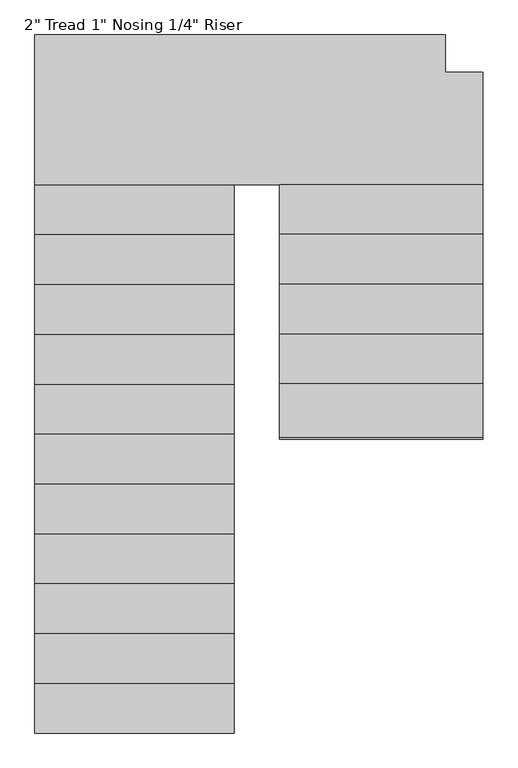
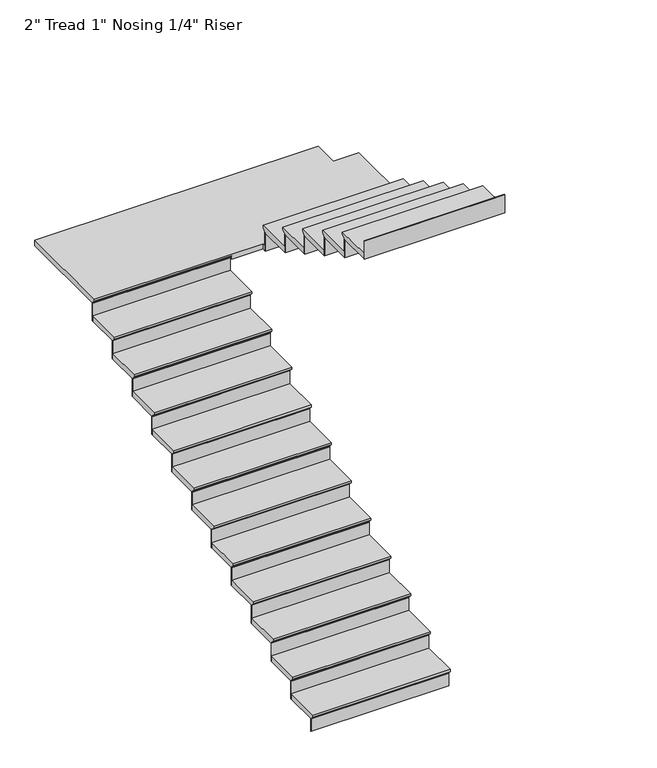
"""IFC4 building model written with IfcOpenShell, lengths in millimetres: stair flight geometry."""

from ifc_helpers import new_model, si_unit, origin, place, context, project, spatial, faceted_brep, source, transform, mapped, element, save


def stair_flight_991562f7(model_context):
    return source(origin(), model_context, "Body", "Brep", [
        faceted_brep([(-1810.3456086, -4300.9794704, 6551.0833333), (-1810.3456086, -4300.9794704, 6570.1333333), (-3029.5456086, -4300.9794704, 6570.1333333), (-3029.5456086, -4300.9794704, 6551.0833333), (-1810.3456086, -4275.5794704, 6525.6833333), (-3029.5456086, -4275.5794704, 6525.6833333), (-1810.3456086, -3970.7794704, 6570.1333333), (-3029.5456086, -3970.7794704, 6570.1333333), (-3029.5456086, -4275.5794704, 6519.3333333), (-3029.5456086, -3970.7794704, 6519.3333333), (-1810.3456086, -3970.7794704, 6519.3333333), (-1810.3456086, -4275.5794704, 6519.3333333)], [[[0, 1, 2, 3]], [[4, 0, 3, 5]], [[2, 1, 6, 7]], [[8, 9, 10, 11]], [[2, 7, 9, 8, 5, 3]], [[8, 11, 4, 5]], [[6, 1, 0, 4, 11, 10]], [[7, 6, 10, 9]]]),
        faceted_brep([(-1810.3456086, -4275.5794704, 6519.3333333), (-1810.3456086, -4275.5794704, 6400.8), (-1810.3456086, -4269.2294704, 6400.8), (-1810.3456086, -4269.2294704, 6519.3333333), (-3029.5456086, -4275.5794704, 6519.3333333), (-3029.5456086, -4269.2294704, 6519.3333333), (-3029.5456086, -4269.2294704, 6400.8), (-3029.5456086, -4275.5794704, 6400.8)], [[[0, 1, 2, 3]], [[4, 5, 6, 7]], [[1, 0, 4, 7]], [[2, 1, 7, 6]], [[3, 2, 6, 5]], [[0, 3, 5, 4]]]),
        faceted_brep([(-1810.3456086, -3970.7794704, 6688.6666667), (-1810.3456086, -3970.7794704, 6519.3333333), (-1810.3456086, -3964.4294704, 6519.3333333), (-1810.3456086, -3964.4294704, 6688.6666667), (-3029.5456086, -3970.7794704, 6688.6666667), (-3029.5456086, -3964.4294704, 6688.6666667), (-3029.5456086, -3964.4294704, 6519.3333333), (-3029.5456086, -3970.7794704, 6519.3333333)], [[[0, 1, 2, 3]], [[4, 5, 6, 7]], [[1, 0, 4, 7]], [[2, 1, 7, 6]], [[3, 2, 6, 5]], [[0, 3, 5, 4]]]),
        faceted_brep([(-3029.5456086, -3996.1794704, 6739.4666667), (-1810.3456086, -3996.1794704, 6739.4666667), (-1810.3456086, -3665.9794704, 6739.4666667), (-3029.5456086, -3665.9794704, 6739.4666667), (-3029.5456086, -3970.7794704, 6688.6666667), (-3029.5456086, -3665.9794704, 6688.6666667), (-1810.3456086, -3665.9794704, 6688.6666667), (-1810.3456086, -3970.7794704, 6688.6666667), (-3029.5456086, -3970.7794704, 6695.0166667), (-3029.5456086, -3996.1794704, 6720.4166667), (-1810.3456086, -3970.7794704, 6695.0166667), (-1810.3456086, -3996.1794704, 6720.4166667)], [[[0, 1, 2, 3]], [[4, 5, 6, 7]], [[0, 3, 5, 4, 8, 9]], [[4, 7, 10, 8]], [[2, 1, 11, 10, 7, 6]], [[3, 2, 6, 5]], [[11, 1, 0, 9]], [[10, 11, 9, 8]]]),
        faceted_brep([(-1810.3456086, -3665.9794704, 6858.0), (-1810.3456086, -3665.9794704, 6688.6666667), (-1810.3456086, -3659.6294704, 6688.6666667), (-1810.3456086, -3659.6294704, 6858.0), (-3029.5456086, -3665.9794704, 6858.0), (-3029.5456086, -3659.6294704, 6858.0), (-3029.5456086, -3659.6294704, 6688.6666667), (-3029.5456086, -3665.9794704, 6688.6666667)], [[[0, 1, 2, 3]], [[4, 5, 6, 7]], [[1, 0, 4, 7]], [[2, 1, 7, 6]], [[3, 2, 6, 5]], [[0, 3, 5, 4]]]),
        faceted_brep([(-3029.5456086, -3691.3794704, 6908.8), (-1810.3456086, -3691.3794704, 6908.8), (-1810.3456086, -3361.1794704, 6908.8), (-3029.5456086, -3361.1794704, 6908.8), (-3029.5456086, -3665.9794704, 6858.0), (-3029.5456086, -3361.1794704, 6858.0), (-1810.3456086, -3361.1794704, 6858.0), (-1810.3456086, -3665.9794704, 6858.0), (-3029.5456086, -3665.9794704, 6864.35), (-3029.5456086, -3691.3794704, 6889.75), (-1810.3456086, -3665.9794704, 6864.35), (-1810.3456086, -3691.3794704, 6889.75)], [[[0, 1, 2, 3]], [[4, 5, 6, 7]], [[0, 3, 5, 4, 8, 9]], [[4, 7, 10, 8]], [[2, 1, 11, 10, 7, 6]], [[3, 2, 6, 5]], [[11, 1, 0, 9]], [[10, 11, 9, 8]]]),
        faceted_brep([(-1810.3456086, -3361.1794704, 7027.3333333), (-1810.3456086, -3361.1794704, 6858.0), (-1810.3456086, -3354.8294704, 6858.0), (-1810.3456086, -3354.8294704, 7027.3333333), (-3029.5456086, -3361.1794704, 7027.3333333), (-3029.5456086, -3354.8294704, 7027.3333333), (-3029.5456086, -3354.8294704, 6858.0), (-3029.5456086, -3361.1794704, 6858.0)], [[[0, 1, 2, 3]], [[4, 5, 6, 7]], [[1, 0, 4, 7]], [[2, 1, 7, 6]], [[3, 2, 6, 5]], [[0, 3, 5, 4]]]),
        faceted_brep([(-3029.5456086, -3386.5794704, 7078.1333333), (-1810.3456086, -3386.5794704, 7078.1333333), (-1810.3456086, -3056.3794704, 7078.1333333), (-3029.5456086, -3056.3794704, 7078.1333333), (-3029.5456086, -3361.1794704, 7027.3333333), (-3029.5456086, -3056.3794704, 7027.3333333), (-1810.3456086, -3056.3794704, 7027.3333333), (-1810.3456086, -3361.1794704, 7027.3333333), (-3029.5456086, -3361.1794704, 7033.6833333), (-3029.5456086, -3386.5794704, 7059.0833333), (-1810.3456086, -3361.1794704, 7033.6833333), (-1810.3456086, -3386.5794704, 7059.0833333)], [[[0, 1, 2, 3]], [[4, 5, 6, 7]], [[0, 3, 5, 4, 8, 9]], [[4, 7, 10, 8]], [[2, 1, 11, 10, 7, 6]], [[3, 2, 6, 5]], [[11, 1, 0, 9]], [[10, 11, 9, 8]]]),
        faceted_brep([(-1810.3456086, -3056.3794704, 7196.6666667), (-1810.3456086, -3056.3794704, 7027.3333333), (-1810.3456086, -3050.0294704, 7027.3333333), (-1810.3456086, -3050.0294704, 7196.6666667), (-3029.5456086, -3056.3794704, 7196.6666667), (-3029.5456086, -3050.0294704, 7196.6666667), (-3029.5456086, -3050.0294704, 7027.3333333), (-3029.5456086, -3056.3794704, 7027.3333333)], [[[0, 1, 2, 3]], [[4, 5, 6, 7]], [[1, 0, 4, 7]], [[2, 1, 7, 6]], [[3, 2, 6, 5]], [[0, 3, 5, 4]]]),
        faceted_brep([(-3029.5456086, -3081.7794704, 7247.4666667), (-1810.3456086, -3081.7794704, 7247.4666667), (-1810.3456086, -2751.5794704, 7247.4666667), (-3029.5456086, -2751.5794704, 7247.4666667), (-3029.5456086, -3056.3794704, 7196.6666667), (-3029.5456086, -2751.5794704, 7196.6666667), (-1810.3456086, -2751.5794704, 7196.6666667), (-1810.3456086, -3056.3794704, 7196.6666667), (-3029.5456086, -3056.3794704, 7203.0166667), (-3029.5456086, -3081.7794704, 7228.4166667), (-1810.3456086, -3056.3794704, 7203.0166667), (-1810.3456086, -3081.7794704, 7228.4166667)], [[[0, 1, 2, 3]], [[4, 5, 6, 7]], [[0, 3, 5, 4, 8, 9]], [[4, 7, 10, 8]], [[2, 1, 11, 10, 7, 6]], [[3, 2, 6, 5]], [[11, 1, 0, 9]], [[10, 11, 9, 8]]]),
        faceted_brep([(-1810.3456086, -2751.5794704, 7366.0), (-1810.3456086, -2751.5794704, 7196.6666667), (-1810.3456086, -2745.2294704, 7196.6666667), (-1810.3456086, -2745.2294704, 7366.0), (-3029.5456086, -2751.5794704, 7366.0), (-3029.5456086, -2745.2294704, 7366.0), (-3029.5456086, -2745.2294704, 7196.6666667), (-3029.5456086, -2751.5794704, 7196.6666667)], [[[0, 1, 2, 3]], [[4, 5, 6, 7]], [[1, 0, 4, 7]], [[2, 1, 7, 6]], [[3, 2, 6, 5]], [[0, 3, 5, 4]]]),
        faceted_brep([(-3029.5456086, -2776.9794704, 7416.8), (-1810.3456086, -2776.9794704, 7416.8), (-1810.3456086, -2446.7794704, 7416.8), (-3029.5456086, -2446.7794704, 7416.8), (-3029.5456086, -2751.5794704, 7366.0), (-3029.5456086, -2446.7794704, 7366.0), (-1810.3456086, -2446.7794704, 7366.0), (-1810.3456086, -2751.5794704, 7366.0), (-3029.5456086, -2751.5794704, 7372.35), (-3029.5456086, -2776.9794704, 7397.75), (-1810.3456086, -2751.5794704, 7372.35), (-1810.3456086, -2776.9794704, 7397.75)], [[[0, 1, 2, 3]], [[4, 5, 6, 7]], [[0, 3, 5, 4, 8, 9]], [[4, 7, 10, 8]], [[2, 1, 11, 10, 7, 6]], [[3, 2, 6, 5]], [[11, 1, 0, 9]], [[10, 11, 9, 8]]]),
        faceted_brep([(-1810.3456086, -2446.7794704, 7535.3333333), (-1810.3456086, -2446.7794704, 7366.0), (-1810.3456086, -2440.4294704, 7366.0), (-1810.3456086, -2440.4294704, 7535.3333333), (-3029.5456086, -2446.7794704, 7535.3333333), (-3029.5456086, -2440.4294704, 7535.3333333), (-3029.5456086, -2440.4294704, 7366.0), (-3029.5456086, -2446.7794704, 7366.0)], [[[0, 1, 2, 3]], [[4, 5, 6, 7]], [[1, 0, 4, 7]], [[2, 1, 7, 6]], [[3, 2, 6, 5]], [[0, 3, 5, 4]]]),
        faceted_brep([(-3029.5456086, -2472.1794704, 7586.1333333), (-1810.3456086, -2472.1794704, 7586.1333333), (-1810.3456086, -2141.9794704, 7586.1333333), (-3029.5456086, -2141.9794704, 7586.1333333), (-3029.5456086, -2446.7794704, 7535.3333333), (-3029.5456086, -2141.9794704, 7535.3333333), (-1810.3456086, -2141.9794704, 7535.3333333), (-1810.3456086, -2446.7794704, 7535.3333333), (-3029.5456086, -2446.7794704, 7541.6833333), (-3029.5456086, -2472.1794704, 7567.0833333), (-1810.3456086, -2446.7794704, 7541.6833333), (-1810.3456086, -2472.1794704, 7567.0833333)], [[[0, 1, 2, 3]], [[4, 5, 6, 7]], [[0, 3, 5, 4, 8, 9]], [[4, 7, 10, 8]], [[2, 1, 11, 10, 7, 6]], [[3, 2, 6, 5]], [[11, 1, 0, 9]], [[10, 11, 9, 8]]]),
        faceted_brep([(-1810.3456086, -2141.9794704, 7704.6666667), (-1810.3456086, -2141.9794704, 7535.3333333), (-1810.3456086, -2135.6294704, 7535.3333333), (-1810.3456086, -2135.6294704, 7704.6666667), (-3029.5456086, -2141.9794704, 7704.6666667), (-3029.5456086, -2135.6294704, 7704.6666667), (-3029.5456086, -2135.6294704, 7535.3333333), (-3029.5456086, -2141.9794704, 7535.3333333)], [[[0, 1, 2, 3]], [[4, 5, 6, 7]], [[1, 0, 4, 7]], [[2, 1, 7, 6]], [[3, 2, 6, 5]], [[0, 3, 5, 4]]]),
        faceted_brep([(-3029.5456086, -2167.3794704, 7755.4666667), (-1810.3456086, -2167.3794704, 7755.4666667), (-1810.3456086, -1837.1794704, 7755.4666667), (-3029.5456086, -1837.1794704, 7755.4666667), (-3029.5456086, -2141.9794704, 7704.6666667), (-3029.5456086, -1837.1794704, 7704.6666667), (-1810.3456086, -1837.1794704, 7704.6666667), (-1810.3456086, -2141.9794704, 7704.6666667), (-3029.5456086, -2141.9794704, 7711.0166667), (-3029.5456086, -2167.3794704, 7736.4166667), (-1810.3456086, -2141.9794704, 7711.0166667), (-1810.3456086, -2167.3794704, 7736.4166667)], [[[0, 1, 2, 3]], [[4, 5, 6, 7]], [[0, 3, 5, 4, 8, 9]], [[4, 7, 10, 8]], [[2, 1, 11, 10, 7, 6]], [[3, 2, 6, 5]], [[11, 1, 0, 9]], [[10, 11, 9, 8]]]),
        faceted_brep([(-1810.3456086, -1837.1794704, 7874.0), (-1810.3456086, -1837.1794704, 7704.6666667), (-1810.3456086, -1830.8294704, 7704.6666667), (-1810.3456086, -1830.8294704, 7874.0), (-3029.5456086, -1837.1794704, 7874.0), (-3029.5456086, -1830.8294704, 7874.0), (-3029.5456086, -1830.8294704, 7704.6666667), (-3029.5456086, -1837.1794704, 7704.6666667)], [[[0, 1, 2, 3]], [[4, 5, 6, 7]], [[1, 0, 4, 7]], [[2, 1, 7, 6]], [[3, 2, 6, 5]], [[0, 3, 5, 4]]]),
        faceted_brep([(-3029.5456086, -1862.5794704, 7924.8), (-1810.3456086, -1862.5794704, 7924.8), (-1810.3456086, -1532.3794704, 7924.8), (-3029.5456086, -1532.3794704, 7924.8), (-3029.5456086, -1837.1794704, 7874.0), (-3029.5456086, -1532.3794704, 7874.0), (-1810.3456086, -1532.3794704, 7874.0), (-1810.3456086, -1837.1794704, 7874.0), (-3029.5456086, -1837.1794704, 7880.35), (-3029.5456086, -1862.5794704, 7905.75), (-1810.3456086, -1837.1794704, 7880.35), (-1810.3456086, -1862.5794704, 7905.75)], [[[0, 1, 2, 3]], [[4, 5, 6, 7]], [[0, 3, 5, 4, 8, 9]], [[4, 7, 10, 8]], [[2, 1, 11, 10, 7, 6]], [[3, 2, 6, 5]], [[11, 1, 0, 9]], [[10, 11, 9, 8]]]),
        faceted_brep([(-1810.3456086, -1532.3794704, 8043.3333333), (-1810.3456086, -1532.3794704, 7874.0), (-1810.3456086, -1526.0294704, 7874.0), (-1810.3456086, -1526.0294704, 8043.3333333), (-3029.5456086, -1532.3794704, 8043.3333333), (-3029.5456086, -1526.0294704, 8043.3333333), (-3029.5456086, -1526.0294704, 7874.0), (-3029.5456086, -1532.3794704, 7874.0)], [[[0, 1, 2, 3]], [[4, 5, 6, 7]], [[1, 0, 4, 7]], [[2, 1, 7, 6]], [[3, 2, 6, 5]], [[0, 3, 5, 4]]]),
        faceted_brep([(-3029.5456086, -1557.7794704, 8094.1333333), (-1810.3456086, -1557.7794704, 8094.1333333), (-1810.3456086, -1227.5794704, 8094.1333333), (-3029.5456086, -1227.5794704, 8094.1333333), (-3029.5456086, -1532.3794704, 8043.3333333), (-3029.5456086, -1227.5794704, 8043.3333333), (-1810.3456086, -1227.5794704, 8043.3333333), (-1810.3456086, -1532.3794704, 8043.3333333), (-3029.5456086, -1532.3794704, 8049.6833333), (-3029.5456086, -1557.7794704, 8075.0833333), (-1810.3456086, -1532.3794704, 8049.6833333), (-1810.3456086, -1557.7794704, 8075.0833333)], [[[0, 1, 2, 3]], [[4, 5, 6, 7]], [[0, 3, 5, 4, 8, 9]], [[4, 7, 10, 8]], [[2, 1, 11, 10, 7, 6]], [[3, 2, 6, 5]], [[11, 1, 0, 9]], [[10, 11, 9, 8]]]),
        faceted_brep([(-1810.3456086, -1227.5794704, 8212.6666667), (-1810.3456086, -1227.5794704, 8043.3333333), (-1810.3456086, -1221.2294704, 8043.3333333), (-1810.3456086, -1221.2294704, 8212.6666667), (-3029.5456086, -1227.5794704, 8212.6666667), (-3029.5456086, -1221.2294704, 8212.6666667), (-3029.5456086, -1221.2294704, 8043.3333333), (-3029.5456086, -1227.5794704, 8043.3333333)], [[[0, 1, 2, 3]], [[4, 5, 6, 7]], [[1, 0, 4, 7]], [[2, 1, 7, 6]], [[3, 2, 6, 5]], [[0, 3, 5, 4]]]),
        faceted_brep([(-3029.5456086, -1252.9794704, 8263.4666667), (-1810.3456086, -1252.9794704, 8263.4666667), (-1810.3456086, -922.7794704, 8263.4666667), (-3029.5456086, -922.7794704, 8263.4666667), (-3029.5456086, -1227.5794704, 8212.6666667), (-3029.5456086, -922.7794704, 8212.6666667), (-1810.3456086, -922.7794704, 8212.6666667), (-1810.3456086, -1227.5794704, 8212.6666667), (-3029.5456086, -1227.5794704, 8219.0166667), (-3029.5456086, -1252.9794704, 8244.4166667), (-1810.3456086, -1227.5794704, 8219.0166667), (-1810.3456086, -1252.9794704, 8244.4166667)], [[[0, 1, 2, 3]], [[4, 5, 6, 7]], [[0, 3, 5, 4, 8, 9]], [[4, 7, 10, 8]], [[2, 1, 11, 10, 7, 6]], [[3, 2, 6, 5]], [[11, 1, 0, 9]], [[10, 11, 9, 8]]]),
        faceted_brep([(-1810.3456086, -922.7794704, 8382.0), (-1810.3456086, -922.7794704, 8212.6666667), (-1810.3456086, -916.4294704, 8212.6666667), (-1810.3456086, -916.4294704, 8382.0), (-3029.5456086, -922.7794704, 8382.0), (-3029.5456086, -916.4294704, 8382.0), (-3029.5456086, -916.4294704, 8212.6666667), (-3029.5456086, -922.7794704, 8212.6666667)], [[[0, 1, 2, 3]], [[4, 5, 6, 7]], [[1, 0, 4, 7]], [[2, 1, 7, 6]], [[3, 2, 6, 5]], [[0, 3, 5, 4]]]),
        faceted_brep([(-289.8083398, -973.5794704, 8432.8), (-289.8083398, -262.3794704, 8432.8), (-518.4083398, -262.3794704, 8432.8), (-518.4083398, -33.7794704, 8432.8), (-3029.5456086, -33.7794704, 8432.8), (-3029.5456086, -948.1794704, 8432.8), (-1534.4083398, -948.1794704, 8432.8), (-1534.4083398, -973.5794704, 8432.8), (-289.8083398, -262.3794704, 8382.0), (-289.8083398, -973.5794704, 8382.0), (-1534.4083398, -973.5794704, 8382.0), (-1534.4083398, -948.1794704, 8382.0), (-1810.3456086, -948.1794704, 8382.0), (-1810.3456086, -922.7794704, 8382.0), (-3029.5456086, -922.7794704, 8382.0), (-3029.5456086, -33.7794704, 8382.0), (-518.4083398, -33.7794704, 8382.0), (-518.4083398, -262.3794704, 8382.0), (-3029.5456086, -922.7794704, 8388.35), (-3029.5456086, -948.1794704, 8413.75), (-1810.3456086, -922.7794704, 8388.35), (-1810.3456086, -948.1794704, 8413.75)], [[[0, 1, 2, 3, 4, 5, 6, 7]], [[8, 9, 10, 11, 12, 13, 14, 15, 16, 17]], [[1, 0, 9, 8]], [[2, 1, 8, 17]], [[3, 2, 17, 16]], [[4, 3, 16, 15]], [[5, 4, 15, 14, 18, 19]], [[14, 13, 20, 18]], [[13, 12, 21, 20]], [[6, 5, 19, 21, 12, 11]], [[7, 6, 11, 10]], [[0, 7, 10, 9]], [[19, 18, 20, 21]]]),
        faceted_brep([(-1534.4083398, -973.5794704, 8551.3333333), (-1534.4083398, -973.5794704, 8382.0), (-1534.4083398, -979.9294704, 8382.0), (-1534.4083398, -979.9294704, 8551.3333333), (-289.8083398, -973.5794704, 8551.3333333), (-289.8083398, -979.9294704, 8551.3333333), (-289.8083398, -979.9294704, 8382.0), (-289.8083398, -973.5794704, 8382.0)], [[[0, 1, 2, 3]], [[4, 5, 6, 7]], [[1, 0, 4, 7]], [[2, 1, 7, 6]], [[3, 2, 6, 5]], [[0, 3, 5, 4]]]),
        faceted_brep([(-289.8083398, -948.1794704, 8602.1333333), (-1534.4083398, -948.1794704, 8602.1333333), (-1534.4083398, -1278.3794704, 8602.1333333), (-289.8083398, -1278.3794704, 8602.1333333), (-289.8083398, -973.5794704, 8551.3333333), (-289.8083398, -1278.3794704, 8551.3333333), (-1534.4083398, -1278.3794704, 8551.3333333), (-1534.4083398, -973.5794704, 8551.3333333), (-289.8083398, -973.5794704, 8557.6833333), (-289.8083398, -948.1794704, 8583.0833333), (-1534.4083398, -973.5794704, 8557.6833333), (-1534.4083398, -948.1794704, 8583.0833333)], [[[0, 1, 2, 3]], [[4, 5, 6, 7]], [[0, 3, 5, 4, 8, 9]], [[4, 7, 10, 8]], [[2, 1, 11, 10, 7, 6]], [[3, 2, 6, 5]], [[11, 1, 0, 9]], [[10, 11, 9, 8]]]),
        faceted_brep([(-1534.4083398, -1278.3794704, 8720.6666667), (-1534.4083398, -1278.3794704, 8551.3333333), (-1534.4083398, -1284.7294704, 8551.3333333), (-1534.4083398, -1284.7294704, 8720.6666667), (-289.8083398, -1278.3794704, 8720.6666667), (-289.8083398, -1284.7294704, 8720.6666667), (-289.8083398, -1284.7294704, 8551.3333333), (-289.8083398, -1278.3794704, 8551.3333333)], [[[0, 1, 2, 3]], [[4, 5, 6, 7]], [[1, 0, 4, 7]], [[2, 1, 7, 6]], [[3, 2, 6, 5]], [[0, 3, 5, 4]]]),
        faceted_brep([(-289.8083398, -1252.9794704, 8771.4666667), (-1534.4083398, -1252.9794704, 8771.4666667), (-1534.4083398, -1583.1794704, 8771.4666667), (-289.8083398, -1583.1794704, 8771.4666667), (-289.8083398, -1278.3794704, 8720.6666667), (-289.8083398, -1583.1794704, 8720.6666667), (-1534.4083398, -1583.1794704, 8720.6666667), (-1534.4083398, -1278.3794704, 8720.6666667), (-289.8083398, -1278.3794704, 8727.0166667), (-289.8083398, -1252.9794704, 8752.4166667), (-1534.4083398, -1278.3794704, 8727.0166667), (-1534.4083398, -1252.9794704, 8752.4166667)], [[[0, 1, 2, 3]], [[4, 5, 6, 7]], [[0, 3, 5, 4, 8, 9]], [[4, 7, 10, 8]], [[2, 1, 11, 10, 7, 6]], [[3, 2, 6, 5]], [[11, 1, 0, 9]], [[10, 11, 9, 8]]]),
        faceted_brep([(-1534.4083398, -1583.1794704, 8890.0), (-1534.4083398, -1583.1794704, 8720.6666667), (-1534.4083398, -1589.5294704, 8720.6666667), (-1534.4083398, -1589.5294704, 8890.0), (-289.8083398, -1583.1794704, 8890.0), (-289.8083398, -1589.5294704, 8890.0), (-289.8083398, -1589.5294704, 8720.6666667), (-289.8083398, -1583.1794704, 8720.6666667)], [[[0, 1, 2, 3]], [[4, 5, 6, 7]], [[1, 0, 4, 7]], [[2, 1, 7, 6]], [[3, 2, 6, 5]], [[0, 3, 5, 4]]]),
        faceted_brep([(-289.8083398, -1557.7794704, 8940.8), (-1534.4083398, -1557.7794704, 8940.8), (-1534.4083398, -1887.9794704, 8940.8), (-289.8083398, -1887.9794704, 8940.8), (-289.8083398, -1583.1794704, 8890.0), (-289.8083398, -1887.9794704, 8890.0), (-1534.4083398, -1887.9794704, 8890.0), (-1534.4083398, -1583.1794704, 8890.0), (-289.8083398, -1583.1794704, 8896.35), (-289.8083398, -1557.7794704, 8921.75), (-1534.4083398, -1583.1794704, 8896.35), (-1534.4083398, -1557.7794704, 8921.75)], [[[0, 1, 2, 3]], [[4, 5, 6, 7]], [[0, 3, 5, 4, 8, 9]], [[4, 7, 10, 8]], [[2, 1, 11, 10, 7, 6]], [[3, 2, 6, 5]], [[11, 1, 0, 9]], [[10, 11, 9, 8]]]),
        faceted_brep([(-1534.4083398, -1887.9794704, 9059.3333333), (-1534.4083398, -1887.9794704, 8890.0), (-1534.4083398, -1894.3294704, 8890.0), (-1534.4083398, -1894.3294704, 9059.3333333), (-289.8083398, -1887.9794704, 9059.3333333), (-289.8083398, -1894.3294704, 9059.3333333), (-289.8083398, -1894.3294704, 8890.0), (-289.8083398, -1887.9794704, 8890.0)], [[[0, 1, 2, 3]], [[4, 5, 6, 7]], [[1, 0, 4, 7]], [[2, 1, 7, 6]], [[3, 2, 6, 5]], [[0, 3, 5, 4]]]),
        faceted_brep([(-289.8083398, -1862.5794704, 9110.1333333), (-1534.4083398, -1862.5794704, 9110.1333333), (-1534.4083398, -2192.7794704, 9110.1333333), (-289.8083398, -2192.7794704, 9110.1333333), (-289.8083398, -1887.9794704, 9059.3333333), (-289.8083398, -2192.7794704, 9059.3333333), (-1534.4083398, -2192.7794704, 9059.3333333), (-1534.4083398, -1887.9794704, 9059.3333333), (-289.8083398, -1887.9794704, 9065.6833333), (-289.8083398, -1862.5794704, 9091.0833333), (-1534.4083398, -1887.9794704, 9065.6833333), (-1534.4083398, -1862.5794704, 9091.0833333)], [[[0, 1, 2, 3]], [[4, 5, 6, 7]], [[0, 3, 5, 4, 8, 9]], [[4, 7, 10, 8]], [[2, 1, 11, 10, 7, 6]], [[3, 2, 6, 5]], [[11, 1, 0, 9]], [[10, 11, 9, 8]]]),
        faceted_brep([(-1534.4083398, -2192.7794704, 9228.6666667), (-1534.4083398, -2192.7794704, 9059.3333333), (-1534.4083398, -2199.1294704, 9059.3333333), (-1534.4083398, -2199.1294704, 9228.6666667), (-289.8083398, -2192.7794704, 9228.6666667), (-289.8083398, -2199.1294704, 9228.6666667), (-289.8083398, -2199.1294704, 9059.3333333), (-289.8083398, -2192.7794704, 9059.3333333)], [[[0, 1, 2, 3]], [[4, 5, 6, 7]], [[1, 0, 4, 7]], [[2, 1, 7, 6]], [[3, 2, 6, 5]], [[0, 3, 5, 4]]]),
        faceted_brep([(-1534.4083398, -2497.5794704, 9398.0), (-1534.4083398, -2497.5794704, 9228.6666667), (-1534.4083398, -2503.9294704, 9228.6666667), (-1534.4083398, -2503.9294704, 9398.0), (-289.8083398, -2497.5794704, 9398.0), (-289.8083398, -2503.9294704, 9398.0), (-289.8083398, -2503.9294704, 9228.6666667), (-289.8083398, -2497.5794704, 9228.6666667)], [[[0, 1, 2, 3]], [[4, 5, 6, 7]], [[1, 0, 4, 7]], [[2, 1, 7, 6]], [[3, 2, 6, 5]], [[0, 3, 5, 4]]]),
        faceted_brep([(-289.8083398, -2167.3794704, 9279.4666667), (-1534.4083398, -2167.3794704, 9279.4666667), (-1534.4083398, -2497.5794704, 9279.4666667), (-289.8083398, -2497.5794704, 9279.4666667), (-289.8083398, -2192.7794704, 9228.6666667), (-289.8083398, -2497.5794704, 9228.6666667), (-1534.4083398, -2497.5794704, 9228.6666667), (-1534.4083398, -2192.7794704, 9228.6666667), (-289.8083398, -2192.7794704, 9235.0166667), (-289.8083398, -2167.3794704, 9260.4166667), (-1534.4083398, -2192.7794704, 9235.0166667), (-1534.4083398, -2167.3794704, 9260.4166667)], [[[0, 1, 2, 3]], [[4, 5, 6, 7]], [[0, 3, 5, 4, 8, 9]], [[4, 7, 10, 8]], [[2, 1, 11, 10, 7, 6]], [[3, 2, 6, 5]], [[11, 1, 0, 9]], [[10, 11, 9, 8]]]),
    ])


if __name__ == "__main__":
    model = new_model("IFC4")
    model_context = context("Model", 3, world=origin())
    ifc_project = project(units=[si_unit("LENGTHUNIT", "METRE", prefix="MILLI")], contexts=[model_context])
    site = spatial("IfcSite", under=ifc_project)
    building = spatial("IfcBuilding", under=site)
    placement = place(None, origin())
    stair_flight_shape = stair_flight_991562f7(model_context)
    element("IfcStairFlight", 1, ObjectType="2\" Tread 1\" Nosing 1/4\" Riser", at=placement, inside=building, context=model_context, shape_type="MappedRepresentation", body=[
        mapped(stair_flight_shape, transform((0.0, 0.0, 0.0), x_axis=(1.0, 0.0, 0.0), y_axis=(0.0, 1.0, 0.0), z_axis=(0.0, 0.0, 1.0))),
    ])
    save(model, "model.ifc")
